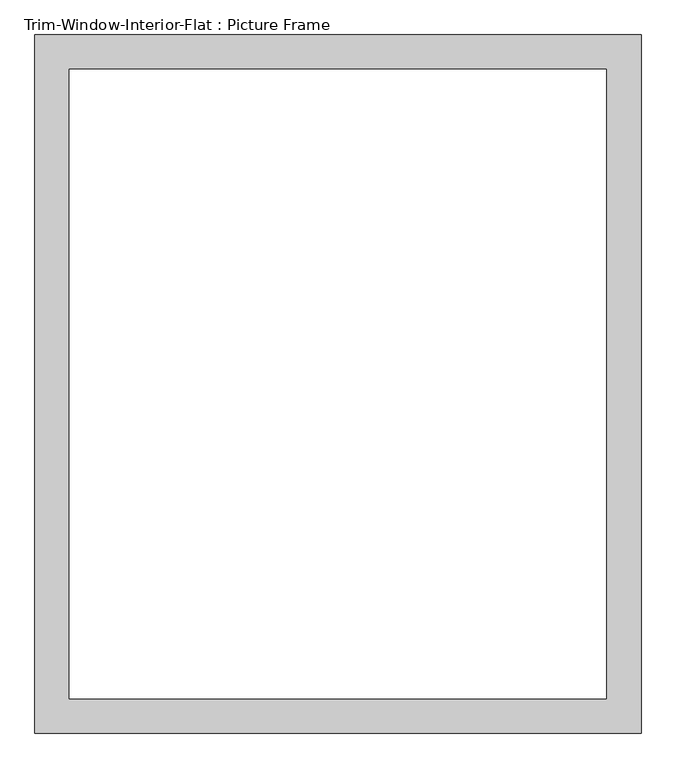
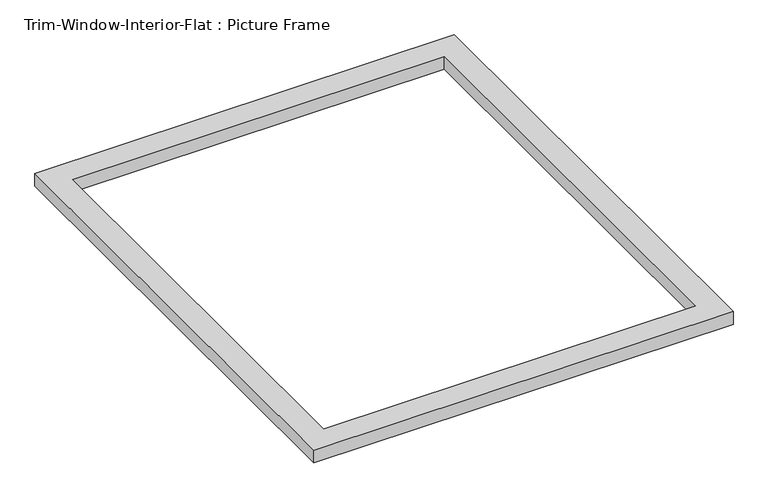
"""IFC4 building model written with IfcOpenShell, lengths in millimetres: proxy geometry, Trim-Window-Interior-Flat : Picture Frame."""

from ifc_helpers import new_model, si_unit, origin, origin_with_axes, place, context, project, spatial, polyline, outline, extrude, source, transform, mapped, element, save


def trim_window_interior_flat_picture_frame_9adb9ca0(model_context):
    return source(origin(), model_context, "Body", "SweptSolid", [
        extrude(outline(polyline([(501.65, -44.45), (-501.65, -44.45), (-501.65, 1111.25), (501.65, 1111.25), (501.65, -44.45)]), holes=[polyline([(444.5, 12.7), (444.5, 1054.1), (-444.5, 1054.1), (-444.5, 12.7), (444.5, 12.7)])]), origin_with_axes(), (0.0, 0.0, 1.0), 31.75),
    ])


if __name__ == "__main__":
    model = new_model("IFC4")
    model_context = context("Model", 3, world=origin())
    ifc_project = project(units=[si_unit("LENGTHUNIT", "METRE", prefix="MILLI")], contexts=[model_context])
    site = spatial("IfcSite", under=ifc_project)
    building = spatial("IfcBuilding", under=site)
    placement = place(None, origin())
    trim_window_interior_flat_picture_frame_shape = trim_window_interior_flat_picture_frame_9adb9ca0(model_context)
    element("IfcBuildingElementProxy", 1, Name="Trim-Window-Interior-Flat : Picture Frame", ObjectType="Trim-Window-Interior-Flat : Picture Frame", at=placement, inside=building, context=model_context, shape_type="MappedRepresentation", body=[
        mapped(trim_window_interior_flat_picture_frame_shape, transform((0.0, 0.0, 0.0), x_axis=(1.0, 0.0, 0.0), y_axis=(0.0, 1.0, 0.0), z_axis=(0.0, 0.0, 1.0))),
    ])
    save(model, "model.ifc")

# Revit data of these elements
# Type "Trim-Window-Interior-Flat : Picture Frame"
#   Trim Thickness_Picture Frame = 0' - 1 1/4"
#   Trim Width = 0' - 2 1/4"
#   Trim Thickness_with Sill = 0' - 0 3/4"
#   Sill Thickness = 0' - 1 1/4"
#   Opening Width [instance default] = 2' - 0"
#   Opening Height [instance default] = 3' - 0"
#   Default Elevation = 4' - 0"
#   Sill = no
#   Picture Frame = yes
#   Trim Material [instance default] = none
# Element 1 (IfcBuildingElementProxy, "Trim-Window-Interior-Flat : Picture Frame")
#   Opening Width = 3' - 0"
#   Opening Height = 3' - 6"
#   Trim Material = Wood - Stained
#   Materials on its faces: "Wood - Stained"
# Materials
#   "Wood - Stained": class "Wood", colour RGB 224 178 126, transparency 0, Cost = 0
